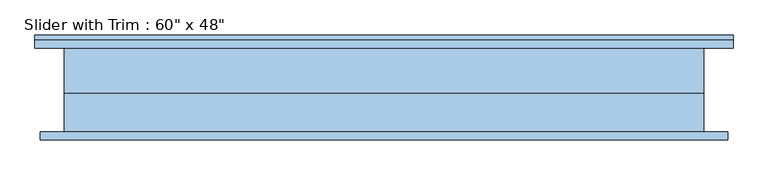
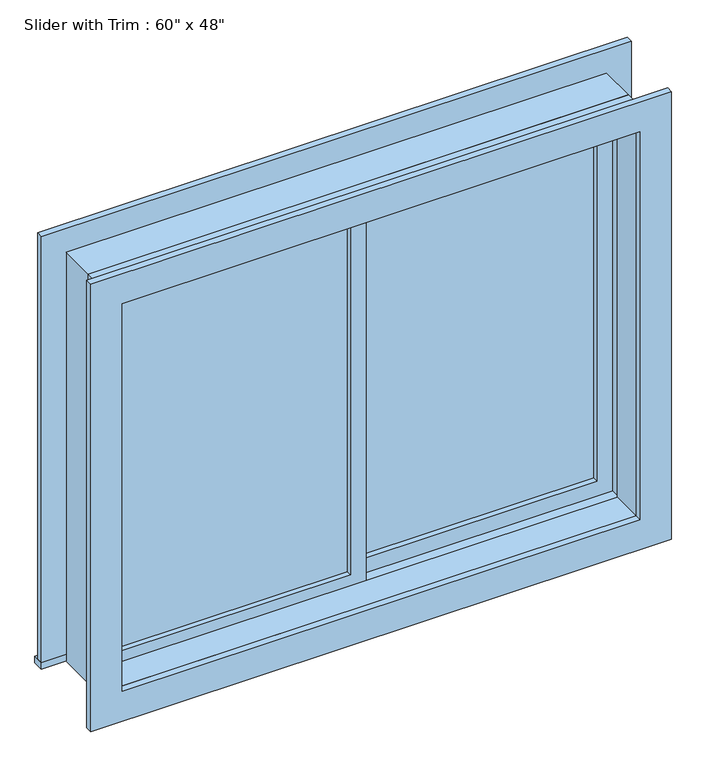
"""IFC4 building model written with IfcOpenShell, lengths in millimetres: window geometry."""

from ifc_helpers import new_model, si_unit, frame, origin, place, context, project, spatial, polyline, outline, extrude, source, transform, mapped, element, save


def window_c4d7a2b1(model_context):
    return source(origin(), model_context, "Body", "SweptSolid", [
        extrude(outline(polyline([(-698.5, 20.625), (-22.225, 20.625), (-22.225, 7.925), (-698.5, 7.925), (-698.5, 20.625)])), frame((0.0, 0.0, 977.9), z_axis=(0.0, 0.0, 1.0), x_axis=(1.0, 0.0, 0.0)), (0.0, 0.0, 1.0), 1092.2),
        extrude(outline(polyline([(2114.55, -742.95), (933.45, -742.95), (933.45, 22.225), (2114.55, 22.225), (2114.55, -742.95)]), holes=[polyline([(2070.1, -698.5), (2070.1, -22.225), (977.9, -22.225), (977.9, -698.5), (2070.1, -698.5)])]), frame((0.0, -7.95, 0.0), z_axis=(0.0, 1.0, 0.0), x_axis=(0.0, 0.0, 1.0)), (0.0, 0.0, 1.0), 44.45),
        extrude(outline(polyline([(-831.85, 131.75), (831.85, 131.75), (831.85, 100.0), (-831.85, 100.0), (-831.85, 131.75)])), frame((0.0, 0.0, 914.4), z_axis=(0.0, 0.0, 1.0), x_axis=(1.0, 0.0, 0.0)), (0.0, 0.0, 1.0), 19.05),
        extrude(outline(polyline([(2114.55, -742.95), (2114.55, 742.95), (933.45, 742.95), (933.45, 831.85), (2203.45, 831.85), (2203.45, -831.85), (933.45, -831.85), (933.45, -742.95), (2114.55, -742.95)])), frame((0.0, 100.0, 0.0), z_axis=(0.0, 1.0, 0.0), x_axis=(0.0, 0.0, 1.0)), (0.0, 0.0, 1.0), 19.05),
        extrude(outline(polyline([(2190.75, 819.15), (2190.75, -819.15), (857.25, -819.15), (857.25, 819.15), (2190.75, 819.15)]), holes=[polyline([(2101.85, 730.25), (946.15, 730.25), (946.15, -730.25), (2101.85, -730.25), (2101.85, 730.25)])]), frame((0.0, -119.05, 0.0), z_axis=(0.0, 1.0, 0.0), x_axis=(0.0, 0.0, 1.0)), (0.0, 0.0, 1.0), 19.05),
        extrude(outline(polyline([(698.5, 52.375), (22.225, 52.375), (22.225, 65.075), (698.5, 65.075), (698.5, 52.375)])), frame((0.0, 0.0, 977.9), z_axis=(0.0, 0.0, 1.0), x_axis=(1.0, 0.0, 0.0)), (0.0, 0.0, 1.0), 1092.2),
        extrude(outline(polyline([(2114.55, -22.225), (933.45, -22.225), (933.45, 742.95), (2114.55, 742.95), (2114.55, -22.225)]), holes=[polyline([(2070.1, 22.225), (2070.1, 698.5), (977.9, 698.5), (977.9, 22.225), (2070.1, 22.225)])]), frame((0.0, 36.5, 0.0), z_axis=(0.0, 1.0, 0.0), x_axis=(0.0, 0.0, 1.0)), (0.0, 0.0, 1.0), 44.45),
        extrude(outline(polyline([(2133.6, -762.0), (914.4, -762.0), (914.4, 762.0), (2133.6, 762.0), (2133.6, -762.0)]), holes=[polyline([(2101.85, -730.25), (2101.85, 730.25), (946.15, 730.25), (946.15, -730.25), (2101.85, -730.25)])]), frame((0.0, -100.0, 0.0), z_axis=(0.0, 1.0, 0.0), x_axis=(0.0, 0.0, 1.0)), (0.0, 0.0, 1.0), 92.05),
        extrude(outline(polyline([(2133.6, 762.0), (2133.6, -762.0), (914.4, -762.0), (914.4, 762.0), (2133.6, 762.0)]), holes=[polyline([(2114.55, 742.95), (933.45, 742.95), (933.45, -742.95), (2114.55, -742.95), (2114.55, 742.95)])]), frame((0.0, -7.95, 0.0), z_axis=(0.0, 1.0, 0.0), x_axis=(0.0, 0.0, 1.0)), (0.0, 0.0, 1.0), 107.95),
    ])


if __name__ == "__main__":
    model = new_model("IFC4")
    model_context = context("Model", 3, world=origin())
    ifc_project = project(units=[si_unit("LENGTHUNIT", "METRE", prefix="MILLI")], contexts=[model_context])
    site = spatial("IfcSite", under=ifc_project)
    building = spatial("IfcBuilding", under=site)
    placement = place(None, origin())
    window_shape = window_c4d7a2b1(model_context)
    element("IfcWindow", 1, ObjectType="Slider with Trim : 60\" x 48\"", at=placement, inside=building, context=model_context, shape_type="MappedRepresentation", body=[
        mapped(window_shape, transform((0.0, 0.0, 0.0), x_axis=(1.0, 0.0, 0.0), y_axis=(0.0, 1.0, 0.0), z_axis=(0.0, 0.0, 1.0))),
    ])
    save(model, "model.ifc")

# Revit data of these elements
# Type "Slider with Trim : 60\" x 48\""
#   Type Mark = "22"
#   Construction Type Id = "GSP4R"
#   Assembly Code = "B2020100"
#   Analytic Construction = "1/8 in Pilkington single glazing"
#   Visual Light Transmittance = 0.9
#   Solar Heat Gain Coefficient = 0.78
#   Heat Transfer Coefficient (U) = 3.6886 W/(m²·K)
#   Height = 1219.2 mm
#   Default Sill Height = 914.4 mm
#   Trim Projection - Ext. = 19.05 mm
#   Trim Projection - Int. = 19.05 mm
#   Trim Width - Exterior = 88.9 mm
#   Trim Width - Interior = 88.9 mm
#   Width = 1524 mm
#   Window Inset = 19.05 mm
#   Define Thermal Properties by = 1
#   Glass Pane Material = Glass
#   Sash Material = Sash
#   Trim Exterior Material = Trim
#   Trim Interior Material = Trim
#   Wall Closure = (empty or 0)
# Element 1 (IfcWindow, "Slider with Trim : 60\" x 48\"")
#   Materials on its faces: "Sash", "Trim", "Glass"
# Materials
#   "Glass": class "Glass", colour RGB 218 227 224, transparency 0.85, Description = "Soda Lime Glass", Cost = 0
#   "Sash": class "Wood", colour RGB 136 99 55, transparency 0
#   "Trim": class "Wood", colour RGB 224 178 126, transparency 0
